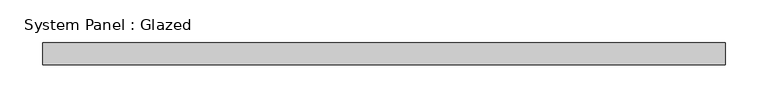
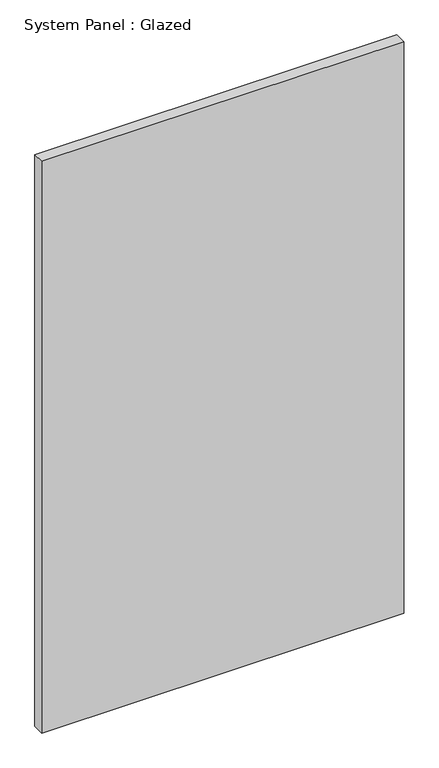
"""IFC4 building model written with IfcOpenShell, lengths in millimetres: plate geometry, System Panel : Glazed."""

from ifc_helpers import new_model, si_unit, origin, origin_with_axes, place, context, project, spatial, polyline, outline, extrude, source, transform, mapped, element, save


def system_panel_glazed_8fb7f6e3(model_context):
    return source(origin(), model_context, "Body", "SweptSolid", [
        extrude(outline(polyline([(396.875, 19.05), (-396.875, 19.05), (-396.875, 44.45), (396.875, 44.45), (396.875, 19.05)])), origin_with_axes(), (0.0, 0.0, 1.0), 1324.8907014),
    ])


if __name__ == "__main__":
    model = new_model("IFC4")
    model_context = context("Model", 3, world=origin())
    ifc_project = project(units=[si_unit("LENGTHUNIT", "METRE", prefix="MILLI")], contexts=[model_context])
    site = spatial("IfcSite", under=ifc_project)
    building = spatial("IfcBuilding", under=site)
    placement = place(None, origin())
    system_panel_glazed_shape = system_panel_glazed_8fb7f6e3(model_context)
    element("IfcPlate", 1, ObjectType="System Panel : Glazed", at=placement, inside=building, context=model_context, shape_type="MappedRepresentation", body=[
        mapped(system_panel_glazed_shape, transform((0.0, 0.0, 0.0), x_axis=(1.0, 0.0, 0.0), y_axis=(0.0, 1.0, 0.0), z_axis=(0.0, 0.0, 1.0))),
    ])
    save(model, "model.ifc")

# Revit data of these elements
# Type "System Panel : Glazed"
#   Construction Type Id = "GSP4R"
#   Analytic Construction = "1/8 in Pilkington single glazing"
#   Visual Light Transmittance = 0.9
#   Solar Heat Gain Coefficient = 0.86
#   Heat Transfer Coefficient (U) = 1.18115 BTU/(h·ft²·°F)
#   Define Thermal Properties by = 1
# Element 1 (IfcPlate, "System Panel : Glazed")
#   Materials on its faces: "Glass"
# Materials
#   "Glass": class "Glass", colour RGB 0 128 192, transparency 0.75, Description = "Soda Lime Glass", Cost = 0
